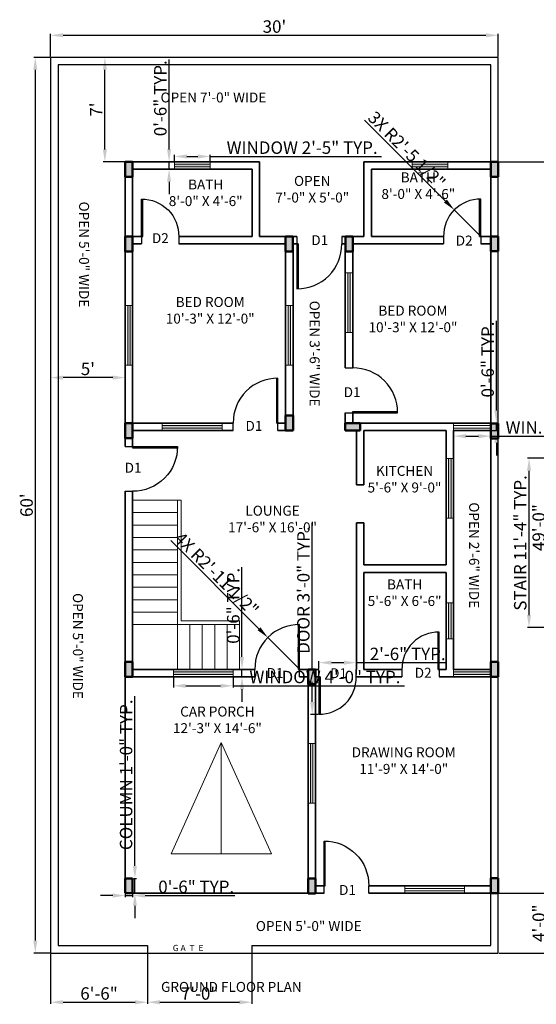
# Model space of a CAD drawing. Units: inches. Extents: x 588 to 1443, y 9704 to 10495.
# Tile 1 of 2: x 588 to 1003, y 9704 to 10495. Entities that reach past the tile are written whole.
import ezdxf

# ---------------------------------------------------------------- set-up
doc = ezdxf.new("R2010")
doc.units = ezdxf.units.IN
for name, color, linetype, lineweight in [('A-ANNO-DIMS', 2, 'Continuous', 18), ('A-ANNO-SYMB', 7, 'Continuous', 18), ('A-ANNO-TEXT', 7, 'Continuous', 25), ('A-AREA-IDEN', 7, 'Continuous', 18), ('A-COLS', 7, 'Continuous', 50), ('A-DOOR', 3, 'Continuous', 25), ('A-DOOR-IDEN', 3, 'Continuous', 18), ('A-FLOR-STRS', 8, 'Continuous', 18), ('A-GLAZ', 4, 'Continuous', 18), ('A-WALL', 7, 'Continuous', 35), ('C-PROP', 8, 'Continuous', 25)]:
    doc.layers.add(name, color=color, linetype=linetype, lineweight=lineweight)
doc.styles.get("Standard").update_dxf_attribs({"font": 'arial.ttf'})
doc.dimstyles.new('ISO-25', dxfattribs={"dimtxt": 10, "dimasz": 10, "dimexe": 1.25, "dimexo": 0.625, "dimtad": 1, "dimdec": 1, "dimlunit": 3, "dimtxsty": 'Standard', "dimcen": 2.5, "dimadec": 0, "dimazin": 0, "dimtfac": 1, "dimtdec": 1, "dimtmove": 0, "dimatfit": 3, "dimfxl": 1, "dimarcsym": 0})

# ---------------------------------------------------------------- blocks, each defined once
blk = doc.blocks.new('*D3')
at = {"layer": 'A-ANNO-DIMS', "color": 0, "lineweight": -2, "transparency": 16777216}
for p, q in [((612.42, 10465.75), (612.42, 10484.09)), ((622.42, 10482.84), (962.42, 10482.84)), ((972.42, 10465.75), (972.42, 10484.09))]:
    blk.add_line(p, q, dxfattribs=at)
at = {"layer": 'A-ANNO-DIMS', "color": 0, "transparency": 16777216}
for points in [[(622.42, 10484.51), (622.42, 10481.17), (612.42, 10482.84)], [(962.42, 10484.51), (962.42, 10481.17), (972.42, 10482.84)]]:
    blk.add_solid(points, dxfattribs=at)
at = {"layer": 'Defpoints', "color": 0, "transparency": 16777216}
for p in [(972.42, 10482.84), (612.42, 10465.12), (972.42, 10465.12)]:
    blk.add_point(p, dxfattribs=at)
at = {"layer": 'A-ANNO-DIMS', "color": 0, "transparency": 16777216, "insert": (792.42, 10488.57), "char_height": 10, "attachment_point": 5}
blk.add_mtext("30'", dxfattribs=at)
blk = doc.blocks.new('*D4')
at = {"layer": 'A-ANNO-DIMS', "color": 0, "lineweight": -2, "transparency": 16777216}
for p, q in [((611.79, 10465.12), (598.86, 10465.12)), ((600.11, 10455.12), (600.11, 9755.12)), ((611.79, 9745.12), (598.86, 9745.12))]:
    blk.add_line(p, q, dxfattribs=at)
at = {"layer": 'A-ANNO-DIMS', "color": 0, "transparency": 16777216}
for points in [[(598.45, 10455.12), (601.78, 10455.12), (600.11, 10465.12)], [(598.45, 9755.12), (601.78, 9755.12), (600.11, 9745.12)]]:
    blk.add_solid(points, dxfattribs=at)
at = {"layer": 'Defpoints', "color": 0, "transparency": 16777216}
for p in [(612.42, 10465.12), (600.11, 9745.12), (612.42, 9745.12)]:
    blk.add_point(p, dxfattribs=at)
at = {"layer": 'A-ANNO-DIMS', "color": 0, "transparency": 16777216, "insert": (594.38, 10105.12), "char_height": 10, "attachment_point": 5, "rotation": 90}
blk.add_mtext("60'", dxfattribs=at)
blk = doc.blocks.new('*D5')
at = {"layer": 'A-ANNO-DIMS', "color": 0, "lineweight": -2, "transparency": 16777216}
for p, q in [((677.79, 10465.12), (654.82, 10465.12)), ((656.07, 10391.12), (656.07, 10455.12)), ((677.79, 10381.12), (654.82, 10381.12))]:
    blk.add_line(p, q, dxfattribs=at)
at = {"layer": 'A-ANNO-DIMS', "color": 0, "transparency": 16777216}
for points in [[(654.41, 10455.12), (657.74, 10455.12), (656.07, 10465.12)], [(654.41, 10391.12), (657.74, 10391.12), (656.07, 10381.12)]]:
    blk.add_solid(points, dxfattribs=at)
at = {"layer": 'Defpoints', "color": 0, "transparency": 16777216}
for p in [(656.07, 10465.12), (678.42, 10465.12), (678.42, 10381.12)]:
    blk.add_point(p, dxfattribs=at)
at = {"layer": 'A-ANNO-DIMS', "color": 0, "transparency": 16777216, "insert": (650.45, 10423.12), "char_height": 10, "attachment_point": 5, "rotation": 90}
blk.add_mtext("7'", dxfattribs=at)
blk = doc.blocks.new('*D6')
at = {"layer": 'A-ANNO-DIMS', "color": 0, "lineweight": -2, "transparency": 16777216}
for p, q in [((612.42, 10217.14), (612.42, 10206.44)), ((672.42, 10217.14), (672.42, 10206.44)), ((662.42, 10207.69), (622.42, 10207.69))]:
    blk.add_line(p, q, dxfattribs=at)
at = {"layer": 'A-ANNO-DIMS', "color": 0, "transparency": 16777216}
for points in [[(622.42, 10209.35), (622.42, 10206.02), (612.42, 10207.69)], [(662.42, 10209.35), (662.42, 10206.02), (672.42, 10207.69)]]:
    blk.add_solid(points, dxfattribs=at)
at = {"layer": 'Defpoints', "color": 0, "transparency": 16777216}
for p in [(612.42, 10217.77), (672.42, 10217.77), (612.42, 10207.69)]:
    blk.add_point(p, dxfattribs=at)
at = {"layer": 'A-ANNO-DIMS', "color": 0, "transparency": 16777216, "insert": (642.42, 10213.4), "char_height": 10, "attachment_point": 5}
blk.add_mtext("5'", dxfattribs=at)
blk = doc.blocks.new('DOOR-SWING-36IN')
for p, q in [((35, 6), (35, 42)), ((36, 6), (36, 42)), ((0, 0), (0, 6)), ((36, 0), (36, 6))]:
    blk.add_line(p, q)
blk.add_arc((35.5, 6.5), 35.5, 89.19307, 180.80693)
blk = doc.blocks.new('DOOR-SWING-30IN')
for p, q in [((0, 30), (0, 36)), ((30, 30), (30, 36)), ((0, 30), (0, 0)), ((1, 30), (1, 0))]:
    blk.add_line(p, q)
blk.add_arc((0.5, 29.5), 29.5, 269.02898, 0.97102)
blk = doc.blocks.new('WIN-48IN')
h = blk.add_hatch(color=256)
h.dxf.hatch_style = 1
h.paths.add_polyline_path([(48, 4), (0, 4), (0, 2), (48, 2)])
for p, q in [((0, 6), (0, 0)), ((0, 4), (48, 4)), ((0, 2), (48, 2)), ((48, 6), (48, 0))]:
    blk.add_line(p, q)
blk = doc.blocks.new('WIN-48IN-OUTLINE')
for p, q in [((0, 6), (0, 0)), ((0, 4), (48, 4)), ((0, 2), (48, 2)), ((48, 6), (48, 0))]:
    blk.add_line(p, q)
blk = doc.blocks.new('WIN-28_8IN')
h = blk.add_hatch(color=256)
h.dxf.hatch_style = 1
h.paths.add_polyline_path([(28.8, 4), (0, 4), (0, 2), (28.8, 2)])
for p, q in [((0, 0), (0, 6)), ((0, 4), (28.8, 4)), ((0, 2), (28.8, 2)), ((28.8, 0), (28.8, 6))]:
    blk.add_line(p, q)
blk = doc.blocks.new('WIN-30IN-OUTLINE')
for p, q in [((0, 0), (0, 6)), ((0, 4), (30, 4)), ((0, 4), (30, 4)), ((0, 2), (30, 2)), ((30, 0), (30, 6))]:
    blk.add_line(p, q)
blk = doc.blocks.new('WIN-30IN')
h = blk.add_hatch(color=256)
h.dxf.hatch_style = 1
h.paths.add_polyline_path([(30, 4), (0, 4), (0, 2), (30, 2)])
for p, q in [((0, 0), (0, 6)), ((0, 4), (30, 4)), ((0, 4), (30, 4)), ((0, 2), (30, 2)), ((30, 0), (30, 6))]:
    blk.add_line(p, q)
blk = doc.blocks.new('COL-6X12IN')
h = blk.add_hatch(color=256)
h.dxf.hatch_style = 1
h.paths.add_polyline_path([(6, 12), (0, 12), (0, 0), (6, 0)])
for p, q in [((0, 12), (6, 12)), ((0, 0), (0, 12)), ((6, 12), (6, 0)), ((6, 0), (0, 0))]:
    blk.add_line(p, q)
blk = doc.blocks.new('STAIR-QUARTER-TURN')
for p, q in [((39, 136), (0, 136)), ((36, 36), (36, 136)), ((39, 39), (39, 136)), ((36, 126), (0, 126)), ((36, 116), (0, 116)), ((36, 106), (0, 106)), ((36, 96), (0, 96)), ((36, 86), (0, 86)), ((36, 76), (0, 76)), ((36, 66), (0, 66)), ((36, 56), (0, 56)), ((36, 46), (0, 46)), ((36, 36), (0, 36)), ((86, 36), (36, 36)), ((36, 36), (36, 0)), ((86, 39), (39, 39)), ((46, 36), (46, 0)), ((56, 36), (56, 0)), ((66, 36), (66, 0)), ((76, 36), (76, 0)), ((86, 39), (86, 0))]:
    blk.add_line(p, q)
blk = doc.blocks.new('*D16')
at = {"layer": 'A-ANNO-DIMS', "color": 0, "lineweight": -2, "transparency": 16777216}
for p, q in [((680.22, 9815.12), (680.22, 9951.63)), ((679.04, 9805.12), (681.47, 9805.12)), ((680.22, 9793.12), (680.22, 9805.12)), ((679.04, 9793.12), (681.47, 9793.12)), ((680.22, 9783.12), (680.22, 9773.12))]:
    blk.add_line(p, q, dxfattribs=at)
at = {"layer": 'A-ANNO-DIMS', "color": 0, "transparency": 16777216}
for points in [[(678.55, 9815.12), (681.88, 9815.12), (680.22, 9805.12)], [(678.55, 9783.12), (681.88, 9783.12), (680.22, 9793.12)]]:
    blk.add_solid(points, dxfattribs=at)
at = {"layer": 'Defpoints', "color": 0, "transparency": 16777216}
for p in [(678.42, 9805.12), (680.22, 9805.12), (678.42, 9793.12)]:
    blk.add_point(p, dxfattribs=at)
at = {"layer": 'A-ANNO-DIMS', "color": 0, "transparency": 16777216, "insert": (674.42, 9888.38), "char_height": 10, "attachment_point": 5, "rotation": 90}
blk.add_mtext('COLUMN 1\'-0" TYP.', dxfattribs=at)
blk = doc.blocks.new('*D17')
at = {"layer": 'A-ANNO-DIMS', "color": 0, "lineweight": -2, "transparency": 16777216}
for p, q in [((662.42, 9791.32), (652.42, 9791.32)), ((672.42, 9792.5), (672.42, 9790.07)), ((672.42, 9791.32), (678.42, 9791.32)), ((678.42, 9792.5), (678.42, 9790.07)), ((688.42, 9791.32), (760.62, 9791.32))]:
    blk.add_line(p, q, dxfattribs=at)
at = {"layer": 'A-ANNO-DIMS', "color": 0, "transparency": 16777216}
for points in [[(662.42, 9792.99), (662.42, 9789.66), (672.42, 9791.32)], [(688.42, 9792.99), (688.42, 9789.66), (678.42, 9791.32)]]:
    blk.add_solid(points, dxfattribs=at)
at = {"layer": 'Defpoints', "color": 0, "transparency": 16777216}
for p in [(672.42, 9793.12), (678.42, 9793.12), (678.42, 9791.32)]:
    blk.add_point(p, dxfattribs=at)
at = {"layer": 'A-ANNO-DIMS', "color": 0, "transparency": 16777216, "insert": (729.52, 9797.05), "char_height": 10, "attachment_point": 5}
blk.add_mtext('0\'-6" TYP.', dxfattribs=at)
blk = doc.blocks.new('*D20')
at = {"layer": 'A-ANNO-DIMS', "color": 0, "lineweight": -2, "transparency": 16777216}
for p, q in [((822.8, 9973.12), (822.8, 10090.62)), ((827.6, 9973.12), (821.55, 9973.12)), ((822.8, 9946.99), (822.8, 9963.12)), ((827.6, 9936.99), (821.55, 9936.99))]:
    blk.add_line(p, q, dxfattribs=at)
at = {"layer": 'A-ANNO-DIMS', "color": 0, "transparency": 16777216}
for points in [[(821.14, 9963.12), (824.47, 9963.12), (822.8, 9973.12)], [(821.14, 9946.99), (824.47, 9946.99), (822.8, 9936.99)]]:
    blk.add_solid(points, dxfattribs=at)
at = {"layer": 'Defpoints', "color": 0, "transparency": 16777216}
for p in [(822.8, 9973.12), (828.22, 9973.12), (828.22, 9936.99)]:
    blk.add_point(p, dxfattribs=at)
at = {"layer": 'A-ANNO-DIMS', "color": 0, "transparency": 16777216, "insert": (817, 10036.87), "char_height": 10, "attachment_point": 5, "rotation": 90}
blk.add_mtext('DOOR 3\'-0" TYP.', dxfattribs=at)
blk = doc.blocks.new('*D21')
at = {"layer": 'A-ANNO-DIMS', "color": 0, "lineweight": -2, "transparency": 16777216}
for p, q in [((828.22, 9973.75), (828.22, 9979.79)), ((838.22, 9978.54), (848.36, 9978.54)), ((858.36, 9973.75), (858.36, 9979.79)), ((858.36, 9978.54), (930.73, 9978.54))]:
    blk.add_line(p, q, dxfattribs=at)
at = {"layer": 'A-ANNO-DIMS', "color": 0, "transparency": 16777216}
for points in [[(838.22, 9980.21), (838.22, 9976.88), (828.22, 9978.54)], [(848.36, 9980.21), (848.36, 9976.88), (858.36, 9978.54)]]:
    blk.add_solid(points, dxfattribs=at)
at = {"layer": 'Defpoints', "color": 0, "transparency": 16777216}
for p in [(828.22, 9973.12), (858.36, 9978.54), (858.36, 9973.12)]:
    blk.add_point(p, dxfattribs=at)
at = {"layer": 'A-ANNO-DIMS', "color": 0, "transparency": 16777216, "insert": (899.55, 9984.27), "char_height": 10, "attachment_point": 5}
blk.add_mtext('2\'-6" TYP.', dxfattribs=at)
blk = doc.blocks.new('*D22')
at = {"layer": 'A-ANNO-DIMS', "color": 0, "lineweight": -2, "transparency": 16777216}
for p, q in [((711.13, 9966.5), (711.13, 9958.67)), ((759.13, 9966.5), (759.13, 9958.67)), ((721.13, 9959.92), (749.13, 9959.92)), ((759.13, 9959.92), (896.92, 9959.92))]:
    blk.add_line(p, q, dxfattribs=at)
at = {"layer": 'A-ANNO-DIMS', "color": 0, "transparency": 16777216}
for points in [[(721.13, 9961.59), (721.13, 9958.26), (711.13, 9959.92)], [(749.13, 9961.59), (749.13, 9958.26), (759.13, 9959.92)]]:
    blk.add_solid(points, dxfattribs=at)
at = {"layer": 'Defpoints', "color": 0, "transparency": 16777216}
for p in [(711.13, 9967.12), (759.13, 9967.12), (759.13, 9959.92)]:
    blk.add_point(p, dxfattribs=at)
at = {"layer": 'A-ANNO-DIMS', "color": 0, "transparency": 16777216, "insert": (833.03, 9965.72), "char_height": 10, "attachment_point": 5}
blk.add_mtext('WINDOW 4\'-0" TYP.', dxfattribs=at)
blk = doc.blocks.new('*D23')
at = {"layer": 'A-ANNO-DIMS', "color": 0, "lineweight": -2, "transparency": 16777216}
for p, q in [((766.33, 9983.12), (766.33, 10055.33)), ((759.76, 9973.12), (767.58, 9973.12)), ((766.33, 9967.12), (766.33, 9973.12)), ((759.76, 9967.12), (767.58, 9967.12)), ((766.33, 9957.12), (766.33, 9947.12))]:
    blk.add_line(p, q, dxfattribs=at)
at = {"layer": 'A-ANNO-DIMS', "color": 0, "transparency": 16777216}
for points in [[(764.67, 9983.12), (768, 9983.12), (766.33, 9973.12)], [(764.67, 9957.12), (768, 9957.12), (766.33, 9967.12)]]:
    blk.add_solid(points, dxfattribs=at)
at = {"layer": 'Defpoints', "color": 0, "transparency": 16777216}
for p in [(759.13, 9973.12), (766.33, 9973.12), (759.13, 9967.12)]:
    blk.add_point(p, dxfattribs=at)
at = {"layer": 'A-ANNO-DIMS', "color": 0, "transparency": 16777216, "insert": (760.6, 10024.23), "char_height": 10, "attachment_point": 5, "rotation": 90}
blk.add_mtext('0\'-6" TYP.', dxfattribs=at)
blk = doc.blocks.new('*D24')
at = {"layer": 'A-ANNO-DIMS', "color": 0, "lineweight": -2, "transparency": 16777216}
for p, q in [((712.02, 10381.75), (712.02, 10386.69)), ((722.02, 10385.44), (730.82, 10385.44)), ((740.82, 10381.75), (740.82, 10386.69)), ((740.82, 10385.44), (878.61, 10385.44))]:
    blk.add_line(p, q, dxfattribs=at)
at = {"layer": 'A-ANNO-DIMS', "color": 0, "transparency": 16777216}
for points in [[(722.02, 10387.11), (722.02, 10383.78), (712.02, 10385.44)], [(730.82, 10387.11), (730.82, 10383.78), (740.82, 10385.44)]]:
    blk.add_solid(points, dxfattribs=at)
at = {"layer": 'Defpoints', "color": 0, "transparency": 16777216}
for p in [(740.82, 10385.44), (712.02, 10381.12), (740.82, 10381.12)]:
    blk.add_point(p, dxfattribs=at)
at = {"layer": 'A-ANNO-DIMS', "color": 0, "transparency": 16777216, "insert": (814.71, 10391.24), "char_height": 10, "attachment_point": 5}
blk.add_mtext('WINDOW 2\'-5" TYP.', dxfattribs=at)
blk = doc.blocks.new('*D25')
at = {"layer": 'A-ANNO-DIMS', "color": 0, "lineweight": -2, "transparency": 16777216}
for p, q in [((707.7, 10391.12), (707.7, 10463.33)), ((711.39, 10381.12), (706.45, 10381.12)), ((707.7, 10375.12), (707.7, 10381.12)), ((711.39, 10375.12), (706.45, 10375.12)), ((707.7, 10365.12), (707.7, 10355.12))]:
    blk.add_line(p, q, dxfattribs=at)
at = {"layer": 'A-ANNO-DIMS', "color": 0, "transparency": 16777216}
for points in [[(706.03, 10391.12), (709.36, 10391.12), (707.7, 10381.12)], [(706.03, 10365.12), (709.36, 10365.12), (707.7, 10375.12)]]:
    blk.add_solid(points, dxfattribs=at)
at = {"layer": 'Defpoints', "color": 0, "transparency": 16777216}
for p in [(707.7, 10381.12), (712.02, 10381.12), (712.02, 10375.12)]:
    blk.add_point(p, dxfattribs=at)
at = {"layer": 'A-ANNO-DIMS', "color": 0, "transparency": 16777216, "insert": (701.97, 10432.23), "char_height": 10, "attachment_point": 5, "rotation": 90}
blk.add_mtext('0\'-6" TYP.', dxfattribs=at)
blk = doc.blocks.new('*D28')
at = {"layer": 'A-ANNO-DIMS', "color": 0, "lineweight": -2, "transparency": 16777216}
for p, q in [((936.42, 10164.5), (936.42, 10159.37)), ((966.42, 10164.5), (966.42, 10159.37)), ((946.42, 10160.62), (956.42, 10160.62)), ((966.42, 10160.62), (1073.95, 10160.62))]:
    blk.add_line(p, q, dxfattribs=at)
at = {"layer": 'A-ANNO-DIMS', "color": 0, "transparency": 16777216}
for points in [[(946.42, 10162.29), (946.42, 10158.96), (936.42, 10160.62)], [(956.42, 10162.29), (956.42, 10158.96), (966.42, 10160.62)]]:
    blk.add_solid(points, dxfattribs=at)
at = {"layer": 'Defpoints', "color": 0, "transparency": 16777216}
for p in [(936.42, 10165.12), (966.42, 10165.12), (966.42, 10160.62)]:
    blk.add_point(p, dxfattribs=at)
at = {"layer": 'A-ANNO-DIMS', "color": 0, "transparency": 16777216, "insert": (1025.18, 10166.35), "char_height": 10, "attachment_point": 5}
blk.add_mtext('WIN. 2\'-6" TYP.', dxfattribs=at)
blk = doc.blocks.new('*D29')
at = {"layer": 'A-ANNO-DIMS', "color": 0, "lineweight": -2, "transparency": 16777216}
for p, q in [((970.92, 10181.12), (970.92, 10253.33)), ((967.04, 10171.12), (972.17, 10171.12)), ((970.92, 10165.12), (970.92, 10171.12)), ((967.04, 10165.12), (972.17, 10165.12)), ((970.92, 10155.12), (970.92, 10145.12))]:
    blk.add_line(p, q, dxfattribs=at)
at = {"layer": 'A-ANNO-DIMS', "color": 0, "transparency": 16777216}
for points in [[(969.25, 10181.12), (972.58, 10181.12), (970.92, 10171.12)], [(969.25, 10155.12), (972.58, 10155.12), (970.92, 10165.12)]]:
    blk.add_solid(points, dxfattribs=at)
at = {"layer": 'Defpoints', "color": 0, "transparency": 16777216}
for p in [(966.42, 10171.12), (970.92, 10171.12), (966.42, 10165.12)]:
    blk.add_point(p, dxfattribs=at)
at = {"layer": 'A-ANNO-DIMS', "color": 0, "transparency": 16777216, "insert": (965.19, 10222.23), "char_height": 10, "attachment_point": 5, "rotation": 90}
blk.add_mtext('0\'-6" TYP.', dxfattribs=at)
blk = doc.blocks.new('*D32')
at = {"layer": 'A-ANNO-DIMS', "color": 0, "lineweight": -2, "transparency": 16777216}
for p, q in [((1016.94, 10142.8), (995.92, 10142.8)), ((997.17, 10016.8), (997.17, 10132.8)), ((1016.94, 10006.8), (995.92, 10006.8))]:
    blk.add_line(p, q, dxfattribs=at)
at = {"layer": 'A-ANNO-DIMS', "color": 0, "transparency": 16777216}
for points in [[(995.5, 10132.8), (998.83, 10132.8), (997.17, 10142.8)], [(995.5, 10016.8), (998.83, 10016.8), (997.17, 10006.8)]]:
    blk.add_solid(points, dxfattribs=at)
at = {"layer": 'Defpoints', "color": 0, "transparency": 16777216}
for p in [(997.17, 10142.8), (1017.57, 10142.8), (1017.57, 10006.8)]:
    blk.add_point(p, dxfattribs=at)
at = {"layer": 'A-ANNO-DIMS', "color": 0, "transparency": 16777216, "insert": (991.37, 10074.8), "char_height": 10, "attachment_point": 5, "rotation": 90}
blk.add_mtext('STAIR 11\'-4" TYP.', dxfattribs=at)
blk = doc.blocks.new('*D34')
at = {"layer": 'A-ANNO-DIMS', "color": 0, "lineweight": -2, "transparency": 16777216}
for p, q in [((967.04, 10381.12), (1013.22, 10381.12)), ((1011.97, 9803.12), (1011.97, 10371.12)), ((967.04, 9793.12), (1013.22, 9793.12))]:
    blk.add_line(p, q, dxfattribs=at)
at = {"layer": 'A-ANNO-DIMS', "color": 0, "transparency": 16777216}
for points in [[(1010.3, 10371.12), (1013.63, 10371.12), (1011.97, 10381.12)], [(1010.3, 9803.12), (1013.63, 9803.12), (1011.97, 9793.12)]]:
    blk.add_solid(points, dxfattribs=at)
at = {"layer": 'Defpoints', "color": 0, "transparency": 16777216}
for p in [(966.42, 10381.12), (1011.97, 10381.12), (966.42, 9793.12)]:
    blk.add_point(p, dxfattribs=at)
at = {"layer": 'A-ANNO-DIMS', "color": 0, "transparency": 16777216, "insert": (1006.24, 10087.12), "char_height": 10, "attachment_point": 5, "rotation": 90}
blk.add_mtext('49\'-0"', dxfattribs=at)
blk = doc.blocks.new('*D35')
at = {"layer": 'A-ANNO-DIMS', "color": 0, "lineweight": -2, "transparency": 16777216}
for p, q in [((967.04, 9793.12), (1013.22, 9793.12)), ((1011.97, 9755.12), (1011.97, 9783.12)), ((973.04, 9745.12), (1013.22, 9745.12))]:
    blk.add_line(p, q, dxfattribs=at)
at = {"layer": 'A-ANNO-DIMS', "color": 0, "transparency": 16777216}
for points in [[(1010.3, 9783.12), (1013.63, 9783.12), (1011.97, 9793.12)], [(1010.3, 9755.12), (1013.63, 9755.12), (1011.97, 9745.12)]]:
    blk.add_solid(points, dxfattribs=at)
at = {"layer": 'Defpoints', "color": 0, "transparency": 16777216}
for p in [(966.42, 9793.12), (1011.97, 9793.12), (972.42, 9745.12)]:
    blk.add_point(p, dxfattribs=at)
at = {"layer": 'A-ANNO-DIMS', "color": 0, "transparency": 16777216, "insert": (1006.24, 9769.12), "char_height": 10, "attachment_point": 5, "rotation": 90}
blk.add_mtext('4\'-0"', dxfattribs=at)
blk = doc.blocks.new('*D36')
at = {"layer": 'A-ANNO-DIMS', "color": 0, "lineweight": -2, "transparency": 16777216}
for p, q in [((612.42, 9744.5), (612.42, 9704.32)), ((690.3, 9750.5), (690.3, 9704.32)), ((622.42, 9705.57), (680.3, 9705.57))]:
    blk.add_line(p, q, dxfattribs=at)
at = {"layer": 'A-ANNO-DIMS', "color": 0, "transparency": 16777216}
for points in [[(622.42, 9707.24), (622.42, 9703.91), (612.42, 9705.57)], [(680.3, 9707.24), (680.3, 9703.91), (690.3, 9705.57)]]:
    blk.add_solid(points, dxfattribs=at)
at = {"layer": 'Defpoints', "color": 0, "transparency": 16777216}
for p in [(690.3, 9751.12), (612.42, 9745.12), (690.3, 9705.57)]:
    blk.add_point(p, dxfattribs=at)
at = {"layer": 'A-ANNO-DIMS', "color": 0, "transparency": 16777216, "insert": (651.36, 9711.3), "char_height": 10, "attachment_point": 5}
blk.add_mtext('6\'-6"', dxfattribs=at)
blk = doc.blocks.new('*D37')
at = {"layer": 'A-ANNO-DIMS', "color": 0, "lineweight": -2, "transparency": 16777216}
for p, q in [((690.3, 9750.5), (690.3, 9704.32)), ((774.3, 9750.5), (774.3, 9704.32)), ((700.3, 9705.57), (764.3, 9705.57))]:
    blk.add_line(p, q, dxfattribs=at)
at = {"layer": 'A-ANNO-DIMS', "color": 0, "transparency": 16777216}
for points in [[(700.3, 9707.24), (700.3, 9703.91), (690.3, 9705.57)], [(764.3, 9707.24), (764.3, 9703.91), (774.3, 9705.57)]]:
    blk.add_solid(points, dxfattribs=at)
at = {"layer": 'Defpoints', "color": 0, "transparency": 16777216}
for p in [(690.3, 9751.12), (774.3, 9751.12), (774.3, 9705.57)]:
    blk.add_point(p, dxfattribs=at)
at = {"layer": 'A-ANNO-DIMS', "color": 0, "transparency": 16777216, "insert": (732.3, 9711.3), "char_height": 10, "attachment_point": 5}
blk.add_mtext('7\'-0"', dxfattribs=at)
blk = doc.blocks.new('*D40')
at = {"layer": 'A-ANNO-DIMS', "color": 0, "lineweight": -2, "transparency": 16777216}
for p, q in [((709.03, 10076.77), (780, 10005.8)), ((812.18, 9973.62), (787.07, 9998.73))]:
    blk.add_line(p, q, dxfattribs=at)
at = {"layer": 'A-ANNO-DIMS', "color": 0, "transparency": 16777216}
blk.add_solid([(781.18, 10006.98), (778.82, 10004.62), (787.07, 9998.73)], dxfattribs=at)
at = {"layer": 'Defpoints', "color": 0, "transparency": 16777216}
for p in [(787.07, 9998.73), (812.18, 9973.62)]:
    blk.add_point(p, dxfattribs=at)
at = {"layer": 'A-ANNO-DIMS', "color": 0, "transparency": 16777216, "insert": (745.08, 10048.92), "char_height": 10, "attachment_point": 5, "rotation": 314.99916}
blk.add_mtext('4X R2\'-11 1/2"', dxfattribs=at)
blk = doc.blocks.new('*D41')
at = {"layer": 'A-ANNO-DIMS', "color": 0, "lineweight": -2, "transparency": 16777216}
for p, q in [((864.8, 10414.74), (929.99, 10349.56)), ((957.92, 10321.62), (937.06, 10342.49))]:
    blk.add_line(p, q, dxfattribs=at)
at = {"layer": 'A-ANNO-DIMS', "color": 0, "transparency": 16777216}
blk.add_solid([(931.17, 10350.74), (928.81, 10348.38), (937.06, 10342.49)], dxfattribs=at)
at = {"layer": 'Defpoints', "color": 0, "transparency": 16777216}
for p in [(937.06, 10342.49), (957.92, 10321.62)]:
    blk.add_point(p, dxfattribs=at)
at = {"layer": 'A-ANNO-DIMS', "color": 0, "transparency": 16777216, "insert": (897.96, 10389.79), "char_height": 10, "attachment_point": 5, "rotation": 314.9996}
blk.add_mtext('3X R2\'-5 1/2"', dxfattribs=at)

msp = doc.modelspace()

# ---------------------------------------------------------------- linework, layer by layer
at = {"layer": 'A-ANNO-SYMB'}
for p, q in [((749.67, 9914.31), (709.27, 9824.77)), ((749.67, 9824.77), (749.67, 9914.31)), ((749.67, 9914.31), (790.07, 9824.77)), ((709.27, 9824.77), (790.07, 9824.77))]:
    msp.add_line(p, q, dxfattribs=at)
at = {"layer": 'A-WALL'}
for p, q in [((780.42, 10381.12), (672.42, 10381.12)), ((672.42, 10152.37), (672.42, 10381.12)), ((780.42, 10321.12), (780.42, 10381.12)), ((966.42, 10381.12), (864.42, 10381.12)), ((864.42, 10321.12), (864.42, 10381.12)), ((774.42, 10375.12), (678.42, 10375.12)), ((678.42, 10321.12), (678.42, 10375.12)), ((774.42, 10321.12), (774.42, 10375.12)), ((966.42, 10375.12), (870.42, 10375.12)), ((870.42, 10321.12), (870.42, 10375.12)), ((966.42, 10321.12), (966.42, 10375.12)), ((686.49, 10321.12), (678.42, 10321.12)), ((774.42, 10321.12), (715.49, 10321.12)), ((810.55, 10321.12), (780.42, 10321.12)), ((864.42, 10321.12), (846.55, 10321.12)), ((928.42, 10321.12), (870.42, 10321.12)), ((966.42, 10321.12), (957.42, 10321.12)), ((678.42, 10171.12), (678.42, 10315.12)), ((685.49, 10315.12), (678.42, 10315.12)), ((774.42, 10315.12), (715.49, 10315.12)), ((801.42, 10315.12), (774.42, 10315.12)), ((801.42, 10171.12), (801.42, 10315.12)), ((807.42, 10165.12), (807.42, 10315.12)), ((811.55, 10315.12), (807.42, 10315.12)), ((849.42, 10315.12), (846.55, 10315.12)), ((849.42, 10215.41), (849.42, 10315.12)), ((870.42, 10315.12), (855.42, 10315.12)), ((855.42, 10215.41), (855.42, 10315.12)), ((928.42, 10315.12), (870.42, 10315.12)), ((966.42, 10315.12), (958.42, 10315.12)), ((966.42, 10171.12), (966.42, 10315.12)), ((849.42, 10165.12), (849.42, 10179.41)), ((855.42, 10171.12), (855.42, 10180.41)), ((759.27, 10171.12), (678.42, 10171.12)), ((801.42, 10171.12), (794.27, 10171.12)), ((966.42, 10171.12), (855.42, 10171.12)), ((759.27, 10165.12), (678.42, 10165.12)), ((678.42, 10151.37), (678.42, 10165.12)), ((807.42, 10165.12), (795.27, 10165.12)), ((858.42, 10165.12), (849.42, 10165.12)), ((858.42, 10121.6), (858.42, 10165.12)), ((930.42, 10165.12), (864.42, 10165.12)), ((864.42, 10121.6), (864.42, 10165.12)), ((930.42, 10057.12), (930.42, 10165.12)), ((966.42, 10165.12), (936.42, 10165.12)), ((936.42, 9973.12), (936.42, 10165.12)), ((966.42, 9973.12), (966.42, 10165.12)), ((672.42, 9793.12), (672.42, 10116.37)), ((678.42, 9973.12), (678.42, 10116.37)), ((858.42, 10121.6), (864.42, 10121.6)), ((858.42, 9973.12), (858.42, 10090.97)), ((858.42, 10090.97), (864.42, 10090.97)), ((864.42, 10057.12), (864.42, 10090.97)), ((930.42, 10057.12), (864.42, 10057.12)), ((864.42, 9973.12), (864.42, 10051.12)), ((930.42, 10051.12), (864.42, 10051.12)), ((930.42, 9973.12), (930.42, 10051.12)), ((776.68, 9973.12), (678.42, 9973.12)), ((819.42, 9973.12), (811.68, 9973.12)), ((819.42, 9973.12), (828.22, 9973.12)), ((858.22, 9973.12), (858.42, 9973.12)), ((894.97, 9973.12), (864.42, 9973.12)), ((930.42, 9973.12), (923.97, 9973.12)), ((966.42, 9973.12), (936.42, 9973.12)), ((776.68, 9967.12), (672.42, 9967.12)), ((819.42, 9967.12), (812.68, 9967.12)), ((819.42, 9793.12), (819.42, 9967.12)), ((825.42, 9799.12), (825.42, 9967.12)), ((825.42, 9967.12), (829.22, 9967.12)), ((858.22, 9967.12), (858.42, 9967.12)), ((894.97, 9967.12), (858.42, 9967.12)), ((966.42, 9967.12), (924.97, 9967.12)), ((966.42, 9799.12), (966.42, 9967.12)), ((833.28, 9799.12), (825.42, 9799.12)), ((966.42, 9799.12), (868.28, 9799.12)), ((832.28, 9793.12), (672.42, 9793.12)), ((966.42, 9793.12), (868.28, 9793.12))]:
    msp.add_line(p, q, dxfattribs=at)
at = {"layer": 'C-PROP'}
for p, q in [((612.42, 10465.12), (612.42, 9745.12)), ((972.42, 10465.12), (612.42, 10465.12)), ((972.42, 9745.12), (972.42, 10465.12)), ((618.42, 10459.12), (618.42, 9751.12)), ((966.42, 10459.12), (618.42, 10459.12)), ((966.42, 10381.12), (966.42, 10459.12)), ((966.42, 9751.12), (966.42, 9793.12)), ((618.42, 9751.12), (690.3, 9751.12)), ((690.3, 9751.12), (690.3, 9745.12)), ((774.3, 9751.12), (774.3, 9745.12)), ((774.3, 9751.12), (966.42, 9751.12)), ((612.42, 9745.12), (690.3, 9745.12)), ((690.3, 9745.12), (972.42, 9745.12))]:
    msp.add_line(p, q, dxfattribs=at)

# ---------------------------------------------------------------- block references
at = {"layer": 'A-COLS'}
for p in [(672.42, 10369.12), (966.42, 10369.08), (672.42, 10309.12), (801.34, 10309.12), (849.48, 10309.12), (966.42, 10309.2), (672.42, 10159.12), (801.42, 10165.12), (966.42, 10158.79), (672.42, 9967.12), (819.42, 9961.12), (966.42, 9967.16), (672.42, 9793.12), (819.42, 9793.06), (966.42, 9793.33)]:
    msp.add_blockref('COL-6X12IN', p, dxfattribs=at)
at = {"layer": 'A-COLS', "rotation": 89.99999999995806}
msp.add_blockref('COL-6X12IN', (861.42, 10165.12), dxfattribs=at)
at = {"layer": 'A-DOOR', "extrusion": (0, 0, -1), "zscale": -1}
for name, p, rotation in [('DOOR-SWING-30IN', (-685.49, 10351.13), 180), ('DOOR-SWING-36IN', (-672.42, 10116.36), 90.00000000000675)]:
    msp.add_blockref(name, p, dxfattribs=dict(at, rotation=rotation))
at = {"layer": 'A-DOOR'}
for name, p, rotation in [('DOOR-SWING-30IN', (958.42, 10351.13), 180), ('DOOR-SWING-36IN', (846.55, 10321.12), 180), ('DOOR-SWING-36IN', (849.42, 10215.41), 270.0000000000084), ('DOOR-SWING-30IN', (924.97, 10003.13), 180)]:
    msp.add_blockref(name, p, dxfattribs=dict(at, rotation=rotation))
for name, p in [('DOOR-SWING-36IN', (759.27, 10165.12)), ('DOOR-SWING-36IN', (776.67, 9967.12)), ('DOOR-SWING-30IN', (828.22, 9937.12))]:
    msp.add_blockref(name, p, dxfattribs=at)
at = {"layer": 'A-DOOR', "extrusion": (0, 0, -1), "zscale": -1}
msp.add_blockref('DOOR-SWING-36IN', (-868.28, 9793.12), dxfattribs=at)
at = {"layer": 'A-FLOR-STRS'}
msp.add_blockref('STAIR-QUARTER-TURN', (678.42, 9973.12), dxfattribs=at)
at = {"layer": 'A-GLAZ'}
for name, p in [('WIN-28_8IN', (712.02, 10375.12)), ('WIN-28_8IN', (903.06, 10375.12)), ('WIN-48IN', (702.26, 10165.12)), ('WIN-30IN-OUTLINE', (936.42, 10165.12)), ('WIN-48IN', (711.13, 9967.12)), ('WIN-30IN', (936.42, 9967.12)), ('WIN-48IN-OUTLINE', (897.23, 9793.12))]:
    msp.add_blockref(name, p, dxfattribs=at)
at = {"layer": 'A-GLAZ', "extrusion": (0, 0, -1), "zscale": -1}
for name, p, rotation in [('WIN-48IN', (-849.42, 10243.85), 89.99999999999596), ('WIN-48IN', (-672.42, 10217.77), 89.99999999999596), ('WIN-48IN', (-801.42, 10217.77), 89.9999999999962), ('WIN-48IN', (-930.42, 10094.78), 89.9999999999955), ('WIN-28_8IN', (-930.42, 9997.77), 90.00000000002433), ('WIN-48IN', (-819.42, 9865.47), 89.99999999999596)]:
    msp.add_blockref(name, p, dxfattribs=dict(at, rotation=rotation))

# ---------------------------------------------------------------- texts
at = {"layer": 'A-ANNO-TEXT', "attachment_point": 1}
for s, width, heights, insert, char_height in [('G A  T  E', 66.6367, [7.18], (710.71, 9751.69), 5), ('{\\fArial|b1|i0|c0|p34;GROUND FLOOR PLAN}', 233.0578, [0], (701.21, 9721.9), 8)]:
    msp.add_mtext_dynamic_manual_height_columns(s, width=width, gutter_width=12.5, heights=heights, dxfattribs=dict(at, insert=insert, char_height=char_height))
at = {"layer": 'A-AREA-IDEN', "char_height": 8, "attachment_point": 1}
for s, width, insert in [('OPEN 7\'-0" WIDE', 203.6948, (700.84, 10436.85)), ('\\pxqc;OPEN\\P7\'-0" X 5\'-0"', 96.8159, (774.42, 10369.77)), ('\\pxqc;BATH\\P8\'-0" X 4\'-6"', 87.4066, (864.42, 10372.63)), ('\\pxqc;BATH\\P8\'-0" X 4\'-6"', 87.4066, (693.45, 10366.91)), ('\\pxqc;BED ROOM\\P10\'-3" X 12\'-0"', 96.8159, (692.36, 10272.45)), ('\\pxqc;BED ROOM\\P10\'-3" X 12\'-0"', 96.8159, (855.42, 10265.5)), ('\\pxqc;KITCHEN\\P5\'-6" X 9\'-0"', 96.8159, (848.6, 10136.69)), ('\\pxqc;LOUNGE\\P17\'-6" X 16\'-0"', 96.8159, (742.51, 10104.68)), ('\\pxqc;BATH\\P5\'-6" X 6\'-6"', 96.8159, (848.71, 10045.44)), ('\\pxqc;CAR PORCH\\P12\'-3" X 14\'-6"', 96.8159, (698.15, 9943.22)), ('\\pxqc;DRAWING ROOM\\P11\'-9" X 14\'-0"', 96.8159, (848, 9910.48)), ('OPEN 5\'-0" WIDE', 203.6948, (777.47, 9770.81))]:
    msp.add_mtext_dynamic_manual_height_columns(s, width=width, gutter_width=12.5, heights=[0], dxfattribs=dict(at, insert=insert))
at = {"layer": 'A-AREA-IDEN', "char_height": 8, "attachment_point": 1, "rotation": 270}
for s, insert in [('OPEN 5\'-0" WIDE', (643.34, 10349.18)), ('OPEN 3\'-6" WIDE', (828.77, 10269.49)), ('OPEN 2\'-6" WIDE', (957, 10107.41)), ('OPEN 5\'-0" WIDE', (638.38, 10034.47))]:
    msp.add_mtext_dynamic_manual_height_columns(s, width=203.6948, gutter_width=12.5, heights=[0], dxfattribs=dict(at, insert=insert))
at = {"layer": 'A-DOOR-IDEN', "char_height": 8, "attachment_point": 1}
for s, insert in [('D2', (693.9, 10323.75)), ('D1', (822.09, 10322.16)), ('D2', (938.24, 10321.83)), ('D1', (848.11, 10199.96)), ('D1', (769.16, 10172.87)), ('D1', (671.99, 10139.23)), ('D1', (786.27, 9974.24)), ('D1', (837.21, 9974.05)), ('D2', (905.23, 9974.39)), ('D1', (844.42, 9799.82))]:
    msp.add_mtext_dynamic_manual_height_columns(s, width=15.8534, gutter_width=12.5, heights=[9.35], dxfattribs=dict(at, insert=insert))

# ---------------------------------------------------------------- dimensions: what is measured, and where the dimension line sits
at = {"layer": 'A-ANNO-DIMS'}
for base, p1, p2, override, picture, middle in [((972.42, 10482.84), (612.42, 10465.12), (972.42, 10465.12), {"dimclrd": 0, "dimclre": 0, "dimclrt": 0}, '*D3', (792.42, 10488.57)), ((612.42, 10207.69), (672.42, 10217.77), (612.42, 10217.77), {"dimclrd": 0, "dimclre": 0, "dimclrt": 0}, '*D6', (642.42, 10213.4)), ((690.3, 9705.57), (612.42, 9745.12), (690.3, 9751.12), {"dimdec": 1, "dimlfac": 1, "dimrnd": 0, "dimzin": 1, "dimdsep": 46, "dimlunit": 4, "dimfrac": 2}, '*D36', (651.36, 9711.3)), ((774.3, 9705.57), (690.3, 9751.12), (774.3, 9751.12), {"dimdec": 1, "dimlfac": 1, "dimrnd": 0, "dimzin": 1, "dimdsep": 46, "dimlunit": 4, "dimfrac": 2}, '*D37', (732.3, 9711.3))]:
    dim = msp.add_linear_dim(base=base, p1=p1, p2=p2, dimstyle='ISO-25', override=override, dxfattribs=at)
    dim.commit()
    dim.dimension.update_dxf_attribs({"geometry": picture, "text_midpoint": middle})
for base, p1, p2, override, picture, middle in [((600.11, 9745.12), (612.42, 10465.12), (612.42, 9745.12), {"dimclrd": 0, "dimclre": 0, "dimclrt": 0}, '*D4', (594.38, 10105.12)), ((656.07, 10465.12), (678.42, 10381.12), (678.42, 10465.12), {"dimclrd": 0, "dimclre": 0, "dimclrt": 0}, '*D5', (650.45, 10423.12)), ((1011.97, 10381.12), (966.42, 9793.12), (966.42, 10381.12), {"dimdec": 1, "dimlfac": 1, "dimrnd": 0, "dimzin": 1, "dimdsep": 46, "dimlunit": 4, "dimfrac": 2}, '*D34', (1006.24, 10087.12)), ((1011.97, 9793.12), (972.42, 9745.12), (966.42, 9793.12), {"dimdec": 1, "dimlfac": 1, "dimrnd": 0, "dimzin": 1, "dimdsep": 46, "dimlunit": 4, "dimfrac": 2}, '*D35', (1006.24, 9769.12))]:
    dim = msp.add_linear_dim(base=base, p1=p1, p2=p2, angle=90, dimstyle='ISO-25', override=override, dxfattribs=at)
    dim.commit()
    dim.dimension.update_dxf_attribs({"geometry": picture, "text_midpoint": middle})
for base, p1, p2, text, picture, middle in [((707.7, 10381.12), (712.02, 10375.12), (712.02, 10381.12), '<> TYP.', '*D25', (701.97, 10432.23)), ((970.92, 10171.12), (966.42, 10165.12), (966.42, 10171.12), '<> TYP.', '*D29', (965.19, 10222.23)), ((997.17, 10142.8), (1017.57, 10006.8), (1017.57, 10142.8), 'STAIR <> TYP.', '*D32', (991.37, 10074.8)), ((822.8, 9973.12), (828.22, 9936.99), (828.22, 9973.12), 'DOOR <> TYP.', '*D20', (817, 10036.87)), ((766.33, 9973.12), (759.13, 9967.12), (759.13, 9973.12), '<> TYP.', '*D23', (760.6, 10024.23)), ((680.22, 9805.12), (678.42, 9793.12), (678.42, 9805.12), 'COLUMN <> TYP.', '*D16', (674.42, 9888.38))]:
    dim = msp.add_linear_dim(base=base, p1=p1, p2=p2, angle=90, text=text, dimstyle='ISO-25', override={"dimdec": 1, "dimlfac": 1, "dimrnd": 0, "dimzin": 1, "dimdsep": 46, "dimlunit": 4, "dimfrac": 2}, dxfattribs=at)
    dim.commit()
    dim.dimension.update_dxf_attribs({"geometry": picture, "text_midpoint": middle})
for center, mpoint, text, picture, middle in [((957.92, 10321.62), (937.06, 10342.49), '3X <>', '*D41', (897.96, 10389.79)), ((812.18, 9973.62), (787.07, 9998.73), '4X <>', '*D40', (745.08, 10048.92))]:
    dim = msp.add_radius_dim(center=center, mpoint=mpoint, text=text, dimstyle='ISO-25', override={"dimdec": 1, "dimlfac": 1, "dimrnd": 0, "dimzin": 1, "dimdsep": 46, "dimlunit": 4, "dimfrac": 2}, dxfattribs=at)
    dim.commit()
    dim.dimension.update_dxf_attribs({"geometry": picture, "text_midpoint": middle})
for base, p1, p2, text, picture, middle in [((740.82, 10385.44), (712.02, 10381.12), (740.82, 10381.12), 'WINDOW <> TYP.', '*D24', (814.71, 10391.24)), ((966.42, 10160.62), (936.42, 10165.12), (966.42, 10165.12), 'WIN. <> TYP.', '*D28', (1025.18, 10166.35)), ((858.36, 9978.54), (828.22, 9973.12), (858.36, 9973.12), '<> TYP.', '*D21', (899.55, 9984.27)), ((759.13, 9959.92), (711.13, 9967.12), (759.13, 9967.12), 'WINDOW <> TYP.', '*D22', (833.03, 9965.72)), ((678.42, 9791.32), (672.42, 9793.12), (678.42, 9793.12), '<> TYP.', '*D17', (729.52, 9797.05))]:
    dim = msp.add_linear_dim(base=base, p1=p1, p2=p2, text=text, dimstyle='ISO-25', override={"dimdec": 1, "dimlfac": 1, "dimrnd": 0, "dimzin": 1, "dimdsep": 46, "dimlunit": 4, "dimfrac": 2}, dxfattribs=at)
    dim.commit()
    dim.dimension.update_dxf_attribs({"geometry": picture, "text_midpoint": middle})

doc.saveas('drawing.dxf')
